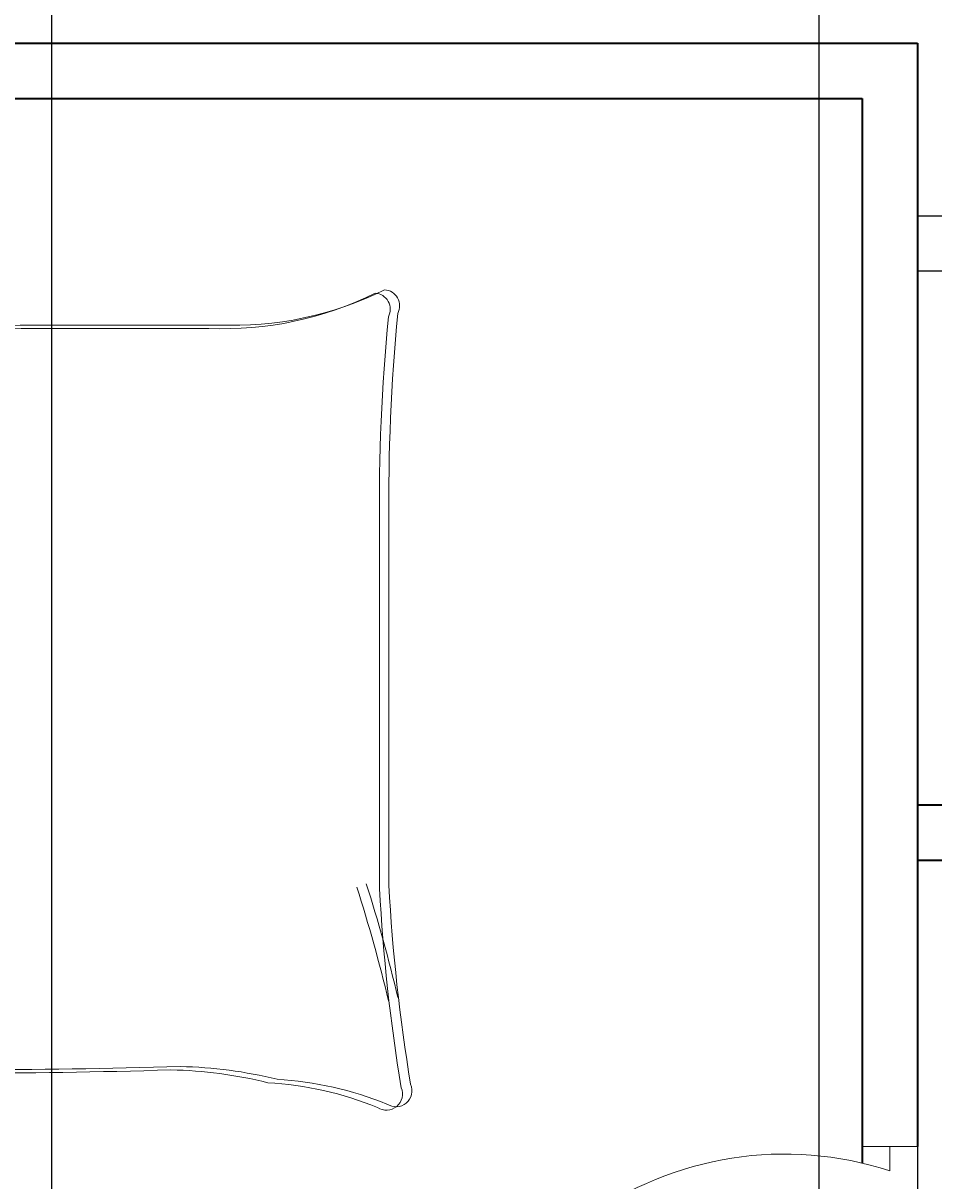
# Model space of a CAD drawing. Units: inches. Extents: x 1088 to 1703, y 668 to 1875.
# Tile 17 of 45: x 1245 to 1319, y 1711 to 1805. Entities that reach past the tile are written whole.
import ezdxf

# ---------------------------------------------------------------- set-up
doc = ezdxf.new("R2010")
doc.units = ezdxf.units.IN
for name, color, linetype, lineweight in [('A-ANNO-DIMS', 2, 'Continuous', 18), ('A-DOOR', 4, 'Continuous', 18), ('A-FLOR-HRAL', 7, 'Continuous', 25), ('A-FURN', 8, 'Continuous', 13), ('A-WALL', 7, 'Continuous', 35)]:
    doc.layers.add(name, color=color, linetype=linetype, lineweight=lineweight)
doc.styles.get("Standard").update_dxf_attribs({"font": 'arial.ttf'})
doc.dimstyles.get("Standard").update_dxf_attribs({"dimtxt": 0.18, "dimasz": 0.18, "dimexe": 0.18, "dimexo": 0.0625, "dimgap": 0.09, "dimtad": 0, "dimtih": 1, "dimtoh": 1, "dimdec": 4, "dimzin": 0, "dimdsep": 46, "dimtxsty": 'Standard', "dimcen": 0.09, "dimadec": 0, "dimazin": 0, "dimtfac": 1, "dimtdec": 4, "dimtofl": 0, "dimtmove": 0, "dimatfit": 3, "dimfxl": 1, "dimtolj": 1, "dimtzin": 0, "dimarcsym": 0})

# ---------------------------------------------------------------- blocks, each defined once
blk = doc.blocks.new('BED-DOUBLE')
for p, q in [((95.003, 18.059), (95.003, 47.568)), ((95.77, 18.333), (95.77, 47.841))]:
    blk.add_line(p, q)
for centre, radius, start, end in [((82.321, 91.302), 27.652, 267.47136, 296.46809), ((83.088, 91.576), 27.652, 267.47136, 296.46809), ((94.554, 65.23), 1.322, 332.65876, 86.02002), ((95.32, 65.504), 1.322, 332.65876, 86.02002), ((254.489, 49.336), 159.496, 174.4998, 180.63509), ((255.256, 49.609), 159.496, 174.4998, 180.63509), ((81.308, -5405.342), 5469.019, 90.002168, 90.286887), ((82.075, -5405.068), 5469.019, 90.002168, 90.286887), ((-28.427, -20.646), 127.629, 13.38322, 17.70533), ((-27.661, -20.372), 127.629, 13.38322, 17.70533), ((240.775, 25.688), 145.971, 182.99578, 189.40907), ((241.542, 25.962), 145.971, 182.99578, 189.40907), ((60.679, 581.233), 578.221, 268.227709, 271.718541), ((61.445, 581.507), 578.221, 268.227709, 271.718541), ((77.344, -32.248), 35.527, 76.06484, 88.91125), ((78.111, -31.975), 35.527, 76.06484, 88.91125), ((84.25, -25.966), 28.247, 67.97508, 86.652), ((85.017, -25.693), 28.247, 67.97508, 86.652), ((96.337, 1.578), 1.306, 236.17358, 23.47814), ((95.57, 1.304), 1.306, 236.17358, 23.47814)]:
    blk.add_arc(centre, radius, start, end)
blk = doc.blocks.new('DOOR-SWING-36')
for p, q in [((36.202, 30.234), (36.202, 28.234)), ((36, 2), (0, 2)), ((36, 0), (36, 2))]:
    blk.add_line(p, q)
blk.add_arc((27.606, 2), 27.606, 71.85834, 180)
blk = doc.blocks.new('*D28')
at = {"layer": 'A-ANNO-DIMS', "color": 0, "lineweight": -2, "transparency": 16777216}
for p, q in [((1170.345, 1803.621), (1170.345, 1857.788)), ((1646.743, 1745.552), (1646.743, 1857.788)), ((1170.525, 1857.608), (1408.147, 1857.608)), ((1646.563, 1857.608), (1408.941, 1857.608))]:
    blk.add_line(p, q, dxfattribs=at)
at = {"layer": 'A-ANNO-DIMS', "color": 0, "transparency": 16777216}
for points in [[(1170.525, 1857.638), (1170.525, 1857.578), (1170.345, 1857.608)], [(1646.563, 1857.638), (1646.563, 1857.578), (1646.743, 1857.608)]]:
    blk.add_solid(points, dxfattribs=at)
at = {"layer": 'Defpoints', "color": 0, "transparency": 16777216}
for p in [(1646.743, 1857.608), (1170.345, 1803.558), (1646.743, 1745.49)]:
    blk.add_point(p, dxfattribs=at)
at = {"layer": 'A-ANNO-DIMS', "color": 0, "transparency": 16777216, "insert": (1408.544, 1857.608), "char_height": 0.18, "attachment_point": 5}
blk.add_mtext('\\A1;476.4', dxfattribs=at)
blk = doc.blocks.new('*D36')
at = {"layer": 'A-ANNO-DIMS', "color": 0, "lineweight": -2, "transparency": 16777216}
for p, q in [((1246.852, 1448.35), (1246.852, 1857.788)), ((1309.352, 1448.35), (1309.352, 1857.788)), ((1247.032, 1857.608), (1277.777, 1857.608)), ((1309.172, 1857.608), (1278.427, 1857.608))]:
    blk.add_line(p, q, dxfattribs=at)
at = {"layer": 'A-ANNO-DIMS', "color": 0, "transparency": 16777216}
for points in [[(1247.032, 1857.638), (1247.032, 1857.578), (1246.852, 1857.608)], [(1309.172, 1857.638), (1309.172, 1857.578), (1309.352, 1857.608)]]:
    blk.add_solid(points, dxfattribs=at)
at = {"layer": 'Defpoints', "color": 0, "transparency": 16777216}
for p in [(1309.352, 1857.608), (1246.852, 1448.287), (1309.352, 1448.287)]:
    blk.add_point(p, dxfattribs=at)
at = {"layer": 'A-ANNO-DIMS', "color": 0, "transparency": 16777216, "insert": (1278.102, 1857.608), "char_height": 0.18, "attachment_point": 5}
blk.add_mtext('\\A1;62.5', dxfattribs=at)
blk = doc.blocks.new('*D38')
at = {"layer": 'A-ANNO-DIMS', "color": 0, "lineweight": -2, "transparency": 16777216}
for p, q in [((1317.345, 1736.945), (1317.345, 725.549)), ((1437.345, 1736.945), (1437.345, 725.549)), ((1317.525, 725.729), (1377.065, 725.729)), ((1437.165, 725.729), (1377.625, 725.729))]:
    blk.add_line(p, q, dxfattribs=at)
at = {"layer": 'A-ANNO-DIMS', "color": 0, "transparency": 16777216}
for points in [[(1317.525, 725.759), (1317.525, 725.699), (1317.345, 725.729)], [(1437.165, 725.759), (1437.165, 725.699), (1437.345, 725.729)]]:
    blk.add_solid(points, dxfattribs=at)
at = {"layer": 'Defpoints', "color": 0, "transparency": 16777216}
for p in [(1317.345, 1737.007), (1437.345, 1737.007), (1437.345, 725.729)]:
    blk.add_point(p, dxfattribs=at)
at = {"layer": 'A-ANNO-DIMS', "color": 0, "transparency": 16777216, "insert": (1377.345, 725.729), "char_height": 0.18, "attachment_point": 5}
blk.add_mtext('\\A1;120', dxfattribs=at)

msp = doc.modelspace()

# ---------------------------------------------------------------- linework, layer by layer
at = {"layer": 'A-DOOR'}
for p, q in [((1312.845, 1713.702), (1317.345, 1713.702)), ((1317.345, 1713.702), (1315.095, 1713.702))]:
    msp.add_line(p, q, dxfattribs=at)
at = {"layer": 'A-FLOR-HRAL'}
for p, q in [((1317.345, 1789.507), (1437.345, 1789.507)), ((1437.345, 1785.007), (1317.345, 1785.007))]:
    msp.add_line(p, q, dxfattribs=at)
at = {"layer": 'A-WALL'}
for p, q in [((1170.345, 1803.558), (1317.345, 1803.558)), ((1170.345, 1803.558), (1317.345, 1803.558)), ((1170.345, 1803.558), (1317.345, 1803.558)), ((1170.345, 1803.558), (1317.345, 1803.558)), ((1170.345, 1803.558), (1317.345, 1803.558)), ((1317.345, 1803.558), (1317.345, 1779.956)), ((1174.845, 1799.058), (1312.845, 1799.058)), ((1312.845, 1799.058), (1312.845, 1712.335)), ((1317.345, 1799.058), (1317.345, 1713.702)), ((1317.345, 1785.007), (1317.345, 1737.007)), ((1345.231, 1741.507), (1317.345, 1741.507)), ((1317.345, 1737.007), (1345.231, 1737.007))]:
    msp.add_line(p, q, dxfattribs=at)

# ---------------------------------------------------------------- block references
at = {"layer": 'A-DOOR'}
msp.add_blockref('DOOR-SWING-36', (1278.893, 1683.468), dxfattribs=at)
at = {"layer": 'A-FURN'}
msp.add_blockref('BED-DOUBLE', (1178.533, 1716.657), dxfattribs=at)

# ---------------------------------------------------------------- dimensions: what is measured, and where the dimension line sits
at = {"layer": 'A-ANNO-DIMS'}
for base, p1, p2, override, picture, middle in [((1646.743, 1857.608), (1170.345, 1803.558), (1646.743, 1745.49), {"dimdec": 1, "dimlfac": 1, "dimrnd": 0, "dimzin": 0, "dimdsep": 46, "dimlunit": 2}, '*D28', (1408.544, 1857.608)), ((1309.352, 1857.608), (1246.852, 1448.287), (1309.352, 1448.287), {"dimdec": 1, "dimlfac": 1, "dimrnd": 0, "dimzin": 0, "dimdsep": 46, "dimlunit": 2}, '*D36', (1278.102, 1857.608)), ((1437.345, 725.729), (1317.345, 1737.007), (1437.345, 1737.007), {"dimdec": 0, "dimlfac": 1, "dimrnd": 0, "dimzin": 0, "dimdsep": 46, "dimlunit": 2}, '*D38', (1377.345, 725.729))]:
    dim = msp.add_linear_dim(base=base, p1=p1, p2=p2, dimstyle='Standard', override=override, dxfattribs=at)
    dim.commit()
    dim.dimension.update_dxf_attribs({"geometry": picture, "text_midpoint": middle})

doc.saveas('drawing.dxf')
